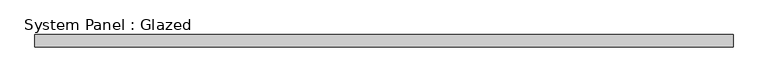
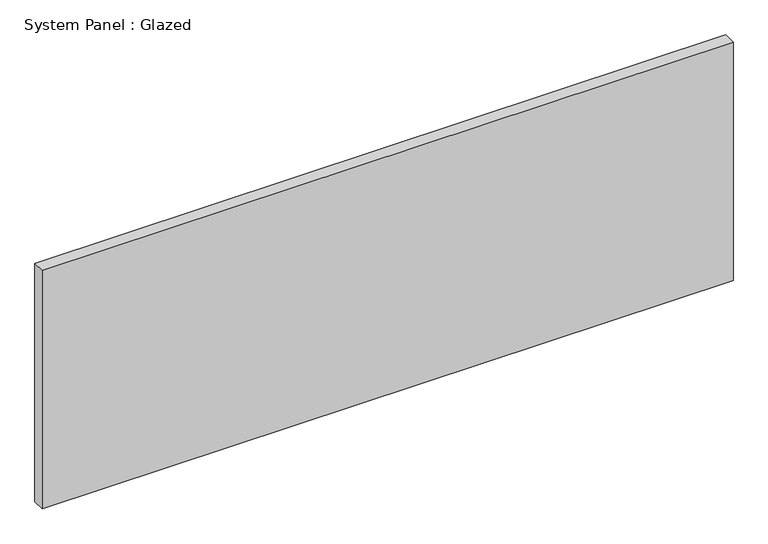
"""IFC4 building model written with IfcOpenShell, lengths in millimetres: plate geometry, System Panel : Glazed."""

from ifc_helpers import new_model, si_unit, origin, origin_with_axes, place, context, project, spatial, polyline, outline, extrude, source, transform, mapped, element, save


def system_panel_glazed_4b614736(model_context):
    return source(origin(), model_context, "Body", "SweptSolid", [
        extrude(outline(polyline([(704.85, 19.05), (-704.85, 19.05), (-704.85, 44.45), (704.85, 44.45), (704.85, 19.05)])), origin_with_axes(), (0.0, 0.0, 1.0), 514.35),
    ])


if __name__ == "__main__":
    model = new_model("IFC4")
    model_context = context("Model", 3, world=origin())
    ifc_project = project(units=[si_unit("LENGTHUNIT", "METRE", prefix="MILLI")], contexts=[model_context])
    site = spatial("IfcSite", under=ifc_project)
    building = spatial("IfcBuilding", under=site)
    placement = place(None, origin())
    system_panel_glazed_shape = system_panel_glazed_4b614736(model_context)
    element("IfcPlate", 1, ObjectType="System Panel : Glazed", at=placement, inside=building, context=model_context, shape_type="MappedRepresentation", body=[
        mapped(system_panel_glazed_shape, transform((0.0, 0.0, 0.0), x_axis=(1.0, 0.0, 0.0), y_axis=(0.0, 1.0, 0.0), z_axis=(0.0, 0.0, 1.0))),
    ])
    save(model, "model.ifc")

# Revit data of these elements
# Type "System Panel : Glazed"
#   Construction Type Id = "GSP4R"
#   Analytic Construction = "1/8 in Pilkington single glazing"
#   Visual Light Transmittance = 0.9
#   Solar Heat Gain Coefficient = 0.86
#   Heat Transfer Coefficient (U) = 1.18115 BTU/(h·ft²·°F)
# Element 1 (IfcPlate, "System Panel : Glazed")
#   Materials on its faces: "Glass"
# Materials
#   "Glass": class "Glass", colour RGB 0 128 192, transparency 0.75, Description = "Soda Lime Glass", Cost = 0
